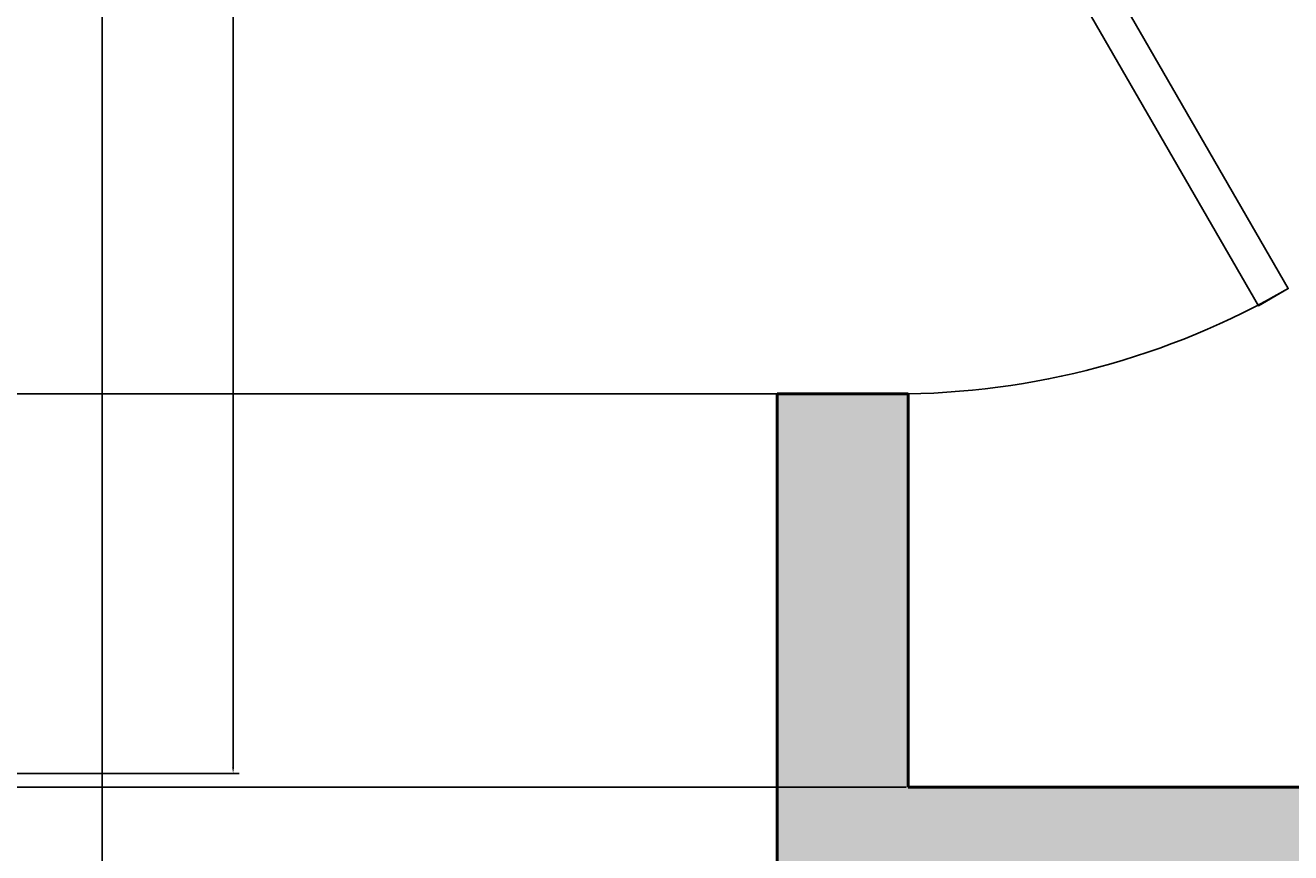
# Model space of a CAD drawing. Units: inches. Extents: x 2231 to 2461, y 2045 to 2455.
# Tile 79 of 95: x 2346 to 2384, y 2333 to 2358. Entities that reach past the tile are written whole.
import ezdxf

# ---------------------------------------------------------------- set-up
doc = ezdxf.new("R2010")
doc.units = ezdxf.units.IN
for name, color, linetype, lineweight in [('A-ANNO-DIMS', 2, 'Continuous', 18), ('A-DOOR', 3, 'Continuous', 25), ('A-WALL', 7, 'Continuous', 50)]:
    doc.layers.add(name, color=color, linetype=linetype, lineweight=lineweight)
doc.layers.add('A-WALL-PATT', color=18, linetype='Continuous', lineweight=13, true_color=0x000000)
doc.styles.get("Standard").update_dxf_attribs({"font": 'arial.ttf'})
doc.dimstyles.get("Standard").update_dxf_attribs({"dimtxt": 0.18, "dimasz": 0.18, "dimexe": 0.18, "dimexo": 0.0625, "dimgap": 0.09, "dimtad": 0, "dimtih": 1, "dimtoh": 1, "dimdec": 4, "dimzin": 0, "dimdsep": 46, "dimtxsty": 'Standard', "dimcen": 0.09, "dimadec": 0, "dimazin": 0, "dimtfac": 1, "dimtdec": 4, "dimtofl": 0, "dimtmove": 0, "dimatfit": 3, "dimfxl": 1, "dimtolj": 1, "dimtzin": 0, "dimarcsym": 0})

# ---------------------------------------------------------------- blocks, each defined once
blk = doc.blocks.new('*U3')
for p, q in [((0, 0), (0, -6)), ((40, 0), (40, -6))]:
    blk.add_line(p, q)
blk.add_lwpolyline([(0, 0), (34.641, 20), (35.516, 18.484), (0.875, -1.516)], close=True)
blk.add_arc((0, 0), 40, 0, 30)
blk = doc.blocks.new('*D20')
at = {"layer": 'A-ANNO-DIMS', "color": 0, "lineweight": -2, "transparency": 16777216}
for p, q in [((2340.251, 2395.253), (2352.368, 2395.253)), ((2352.188, 2395.073), (2352.188, 2365.435)), ((2352.188, 2335.433), (2352.188, 2365.071)), ((2340.251, 2335.253), (2352.368, 2335.253))]:
    blk.add_line(p, q, dxfattribs=at)
at = {"layer": 'A-ANNO-DIMS', "color": 0, "transparency": 16777216}
for points in [[(2352.158, 2395.073), (2352.218, 2395.073), (2352.188, 2395.253)], [(2352.158, 2335.433), (2352.218, 2335.433), (2352.188, 2335.253)]]:
    blk.add_solid(points, dxfattribs=at)
at = {"layer": 'Defpoints', "color": 0, "transparency": 16777216}
for p in [(2340.188, 2395.253), (2352.188, 2395.253), (2340.188, 2335.253)]:
    blk.add_point(p, dxfattribs=at)
at = {"layer": 'A-ANNO-DIMS', "color": 0, "transparency": 16777216, "insert": (2352.188, 2365.253), "char_height": 0.18, "attachment_point": 5}
blk.add_mtext('\\A1;60', dxfattribs=at)
blk = doc.blocks.new('*D53')
at = {"layer": 'A-ANNO-DIMS', "color": 0, "lineweight": -2, "transparency": 16777216}
for p, q in [((2372.731, 2346.833), (2230.981, 2346.833)), ((2231.161, 2346.653), (2231.161, 2341.013)), ((2231.161, 2335.013), (2231.161, 2340.652)), ((2372.731, 2334.833), (2230.981, 2334.833))]:
    blk.add_line(p, q, dxfattribs=at)
at = {"layer": 'A-ANNO-DIMS', "color": 0, "transparency": 16777216}
for points in [[(2231.131, 2346.653), (2231.191, 2346.653), (2231.161, 2346.833)], [(2231.131, 2335.013), (2231.191, 2335.013), (2231.161, 2334.833)]]:
    blk.add_solid(points, dxfattribs=at)
at = {"layer": 'Defpoints', "color": 0, "transparency": 16777216}
for p in [(2231.161, 2346.833), (2372.794, 2346.833), (2372.794, 2334.833)]:
    blk.add_point(p, dxfattribs=at)
at = {"layer": 'A-ANNO-DIMS', "color": 0, "transparency": 16777216, "insert": (2231.161, 2340.833), "char_height": 0.18, "attachment_point": 5}
blk.add_mtext('\\A1;12', dxfattribs=at)
blk = doc.blocks.new('*D54')
at = {"layer": 'A-ANNO-DIMS', "color": 0, "lineweight": -2, "transparency": 16777216}
for p, q in [((2372.731, 2370.833), (2230.981, 2370.833)), ((2231.161, 2370.653), (2231.161, 2359.013)), ((2231.161, 2347.013), (2231.161, 2358.652)), ((2372.731, 2346.833), (2230.981, 2346.833))]:
    blk.add_line(p, q, dxfattribs=at)
at = {"layer": 'A-ANNO-DIMS', "color": 0, "transparency": 16777216}
for points in [[(2231.131, 2370.653), (2231.191, 2370.653), (2231.161, 2370.833)], [(2231.131, 2347.013), (2231.191, 2347.013), (2231.161, 2346.833)]]:
    blk.add_solid(points, dxfattribs=at)
at = {"layer": 'Defpoints', "color": 0, "transparency": 16777216}
for p in [(2231.161, 2370.833), (2372.794, 2370.833), (2372.794, 2346.833)]:
    blk.add_point(p, dxfattribs=at)
at = {"layer": 'A-ANNO-DIMS', "color": 0, "transparency": 16777216, "insert": (2231.161, 2358.833), "char_height": 0.18, "attachment_point": 5}
blk.add_mtext('\\A1;24', dxfattribs=at)
blk = doc.blocks.new('*D66')
at = {"layer": 'A-ANNO-DIMS', "color": 0, "lineweight": -2, "transparency": 16777216}
for p, q in [((2348.189, 2096.895), (2348.189, 2454.645)), ((2408.794, 2096.895), (2408.794, 2454.645)), ((2348.369, 2454.465), (2378.167, 2454.465)), ((2408.614, 2454.465), (2378.815, 2454.465))]:
    blk.add_line(p, q, dxfattribs=at)
at = {"layer": 'A-ANNO-DIMS', "color": 0, "transparency": 16777216}
for points in [[(2348.369, 2454.495), (2348.369, 2454.435), (2348.189, 2454.465)], [(2408.614, 2454.495), (2408.614, 2454.435), (2408.794, 2454.465)]]:
    blk.add_solid(points, dxfattribs=at)
at = {"layer": 'Defpoints', "color": 0, "transparency": 16777216}
for p in [(2408.794, 2454.465), (2348.189, 2096.833), (2408.794, 2096.833)]:
    blk.add_point(p, dxfattribs=at)
at = {"layer": 'A-ANNO-DIMS', "color": 0, "transparency": 16777216, "insert": (2378.491, 2454.465), "char_height": 0.18, "attachment_point": 5}
blk.add_mtext('\\A1;60.6', dxfattribs=at)

msp = doc.modelspace()

# ---------------------------------------------------------------- hatches: boundary and pattern name
at = {"layer": 'A-WALL-PATT'}
h = msp.add_hatch(color=256, dxfattribs=at)
h.dxf.hatch_style = 1
h.paths.add_polyline_path([(2441.7935, 2269.1535), (2432.7935, 2269.1535), (2432.7935, 2186.8328), (2396.7935, 2186.8328), (2396.7935, 2286.8328), (2394.7935, 2286.8328), (2394.7935, 2186.8328), (2334.7935, 2186.8328), (2334.7935, 2182.8328), (2432.7935, 2182.8328), (2432.7935, 2072.8328), (2416.6639, 2072.8328), (2416.6639, 2063.8328), (2441.7935, 2063.8328)])
h.paths.add_polyline_path([(2368.6639, 2072.8328), (2367.04, 2072.8328), (2330.7942, 2072.8328), (2330.7397, 2063.8328), (2368.6639, 2063.8328)])
h.paths.add_polyline_path([(2300.7392, 2068.3328), (2300.7392, 2072.8328), (2298.7935, 2072.8328), (2294.7935, 2072.8328), (2258.7935, 2072.8328), (2258.7935, 2120.8328), (2294.7935, 2120.8328), (2298.7935, 2120.8328), (2298.7935, 2128.8328), (2294.7935, 2128.8328), (2294.7935, 2124.8328), (2258.7935, 2124.8328), (2258.7935, 2182.8328), (2294.7935, 2182.8328), (2294.7935, 2174.8328), (2298.7935, 2174.8328), (2298.7935, 2182.8328), (2304.7935, 2182.8328), (2304.7935, 2186.8328), (2258.7935, 2186.8328), (2258.7935, 2221.999), (2249.7935, 2221.999), (2249.7935, 2063.8328), (2300.7392, 2063.8328)])
h.paths.add_polyline_path([(2391.9338, 2435.8328), (2333.82, 2435.8328), (2333.82, 2426.8328), (2368.7935, 2426.8328), (2368.7935, 2374.9508), (2368.7935, 2370.8328), (2372.3935, 2370.8328), (2372.7935, 2370.8328), (2372.7935, 2426.8328), (2391.9338, 2426.8328)])
h.paths.add_polyline_path([(2441.7935, 2435.8328), (2415.9338, 2435.8328), (2415.9338, 2426.8328), (2432.7935, 2426.8328), (2432.7935, 2334.8328), (2372.7935, 2334.8328), (2372.7935, 2346.8328), (2368.7935, 2346.8328), (2368.7935, 2306.8328), (2360.7935, 2306.8328), (2360.7935, 2302.8328), (2368.7935, 2302.8328), (2372.7935, 2302.8328), (2372.7935, 2330.8328), (2432.7935, 2330.8328), (2432.7935, 2317.1535), (2441.7935, 2317.1535)])
h.paths.add_polyline_path([(2285.82, 2435.8328), (2249.7935, 2435.8328), (2249.7935, 2269.999), (2258.7935, 2269.999), (2258.7935, 2302.8328), (2318.8168, 2302.8328), (2330.7935, 2302.8328), (2330.7935, 2306.8328), (2258.7935, 2306.8328), (2258.7935, 2426.8328), (2285.82, 2426.8328)])

# ---------------------------------------------------------------- linework, layer by layer
at = {"layer": 'A-WALL'}
for p, q in [((2372.7935, 2346.8328), (2368.7935, 2346.8328)), ((2368.7935, 2346.8328), (2368.7935, 2306.8328)), ((2372.7935, 2346.8328), (2372.7935, 2334.8328)), ((2372.7935, 2334.8328), (2432.7935, 2334.8328))]:
    msp.add_line(p, q, dxfattribs=at)

# ---------------------------------------------------------------- block references
at = {"layer": 'A-DOOR', "xscale": 0.6, "yscale": 0.6, "zscale": 0.6, "rotation": 270}
msp.add_blockref('*U3', (2372.3935, 2370.8328), dxfattribs=at)

# ---------------------------------------------------------------- dimensions: what is measured, and where the dimension line sits
at = {"layer": 'A-ANNO-DIMS'}
dim = msp.add_linear_dim(base=(2408.7935, 2454.4653), p1=(2348.1888, 2096.8328), p2=(2408.7935, 2096.8328), dimstyle='Standard', override={"dimdec": 1, "dimlfac": 1, "dimrnd": 0, "dimzin": 0, "dimdsep": 46, "dimlunit": 2}, dxfattribs=at)
dim.commit()
dim.dimension.update_dxf_attribs({"geometry": '*D66', "text_midpoint": (2378.4912, 2454.4653)})
for base, p1, p2, picture, middle in [((2352.1882, 2395.2534), (2340.1882, 2335.2534), (2340.1882, 2395.2534), '*D20', (2352.1882, 2365.2534)), ((2231.161, 2370.8328), (2372.7935, 2346.8328), (2372.7935, 2370.8328), '*D54', (2231.161, 2358.8328)), ((2231.161, 2346.8328), (2372.7935, 2334.8328), (2372.7935, 2346.8328), '*D53', (2231.161, 2340.8328))]:
    dim = msp.add_linear_dim(base=base, p1=p1, p2=p2, angle=90, dimstyle='Standard', override={"dimdec": 0, "dimlfac": 1, "dimrnd": 0, "dimzin": 0, "dimdsep": 46, "dimlunit": 2}, dxfattribs=at)
    dim.commit()
    dim.dimension.update_dxf_attribs({"geometry": picture, "text_midpoint": middle})

doc.saveas('drawing.dxf')
